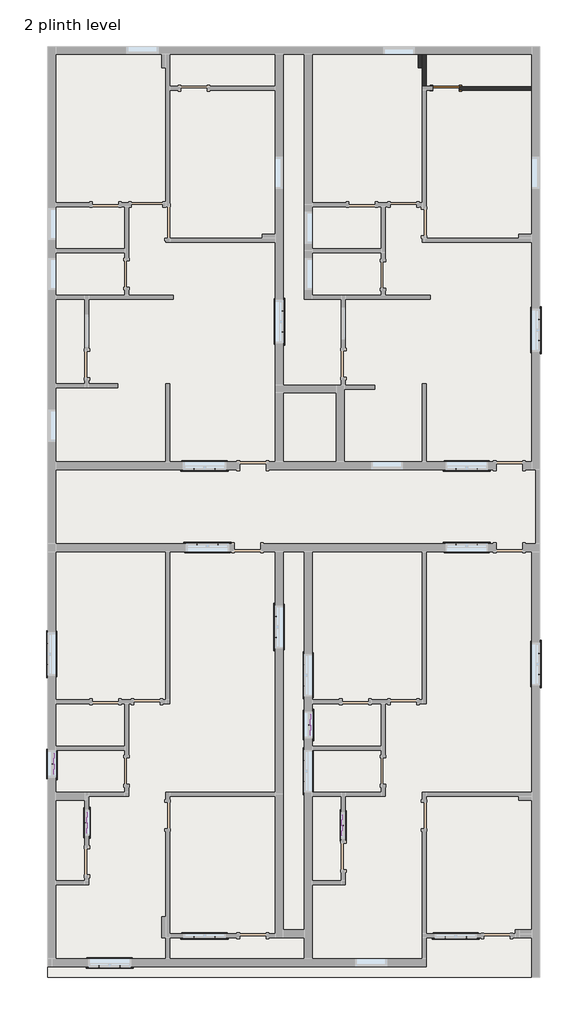
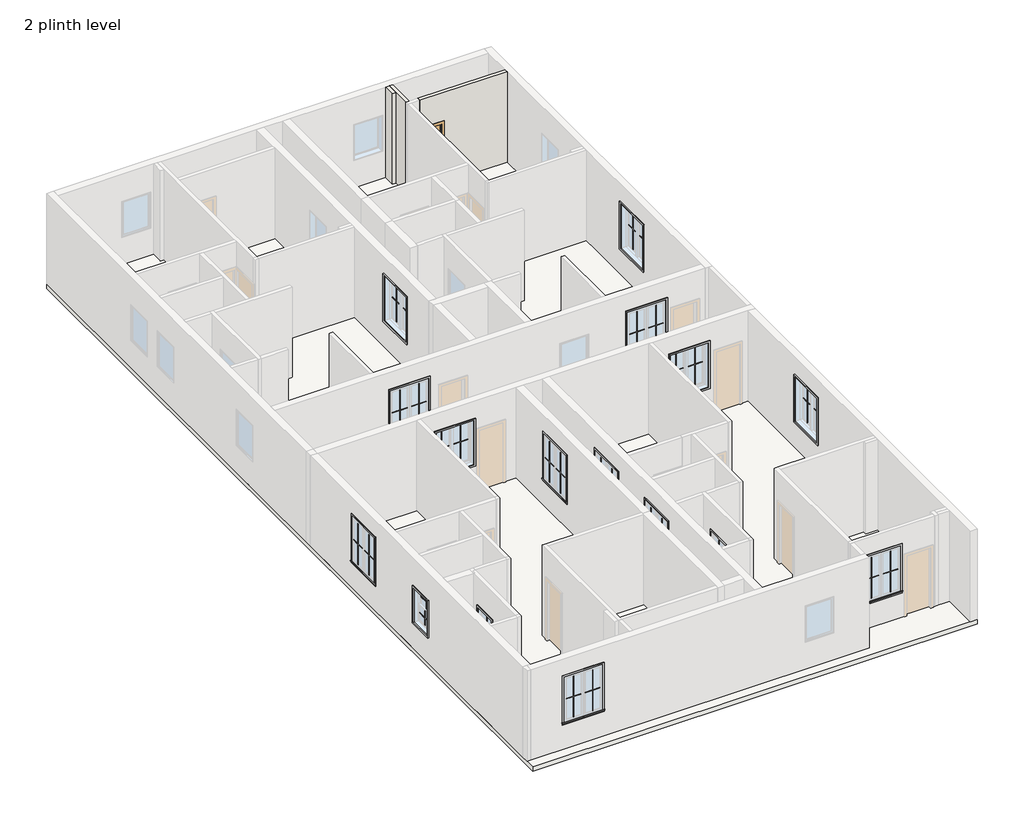
# One storey, part 4 of 4: 72 proxies, 3 walls, 1 door, 1 slab.
"""IFC4 building model written with IfcOpenShell, lengths in millimetres."""

from ifc_helpers import new_model, si_unit, frame, origin, place, context, project, spatial, polyline, outline, extrude, faceted_brep, transform, mapped, element, save
from components import muntin_pattern_2x2_muntin_pattern_2x2_6dad3731, muntin_pattern_2x2_muntin_pattern_2x2_a30a3345, muntin_pattern_2x2_muntin_pattern_2x2_b8ba09c9, trim_window_exterior_flat_with_sill_92b9b949, trim_window_exterior_flat_with_sill_6cd3ad68, trim_window_interior_flat_picture_frame_3bb882cf, trim_window_interior_flat_picture_frame_840a62db, door_f2b275c1

model = new_model("IFC4")

# Units and contexts
model_context = context("Model", 3, world=origin())
ifc_project = project(units=[si_unit("LENGTHUNIT", "METRE", prefix="MILLI")], contexts=[model_context])

# Site, building, storey
site = spatial("IfcSite", under=ifc_project)
building = spatial("IfcBuilding", under=site)
storey = spatial("IfcBuildingStorey", under=building, Name="2 plinth level", Elevation=457.2)

# Proxies
placement = place(None, origin())
muntin_pattern_2x2_muntin_pattern_2x2_shape = muntin_pattern_2x2_muntin_pattern_2x2_6dad3731(model_context)
element("IfcBuildingElementProxy", 1, Name="Muntin Pattern_2x2 : Muntin Pattern_2x2", ObjectType="Muntin Pattern_2x2 : Muntin Pattern_2x2", at=placement, inside=storey, context=model_context, shape_type="MappedRepresentation", body=[
    mapped(muntin_pattern_2x2_muntin_pattern_2x2_shape, transform((-8343.3525468, -3788.9429449, 1441.45), x_axis=(0.0, 1.0, 0.0), y_axis=(-1.0, 0.0, 0.0), z_axis=(0.0, 0.0, 1.0))),
])
element("IfcBuildingElementProxy", 2, Name="Muntin Pattern_2x2 : Muntin Pattern_2x2", ObjectType="Muntin Pattern_2x2 : Muntin Pattern_2x2", at=placement, inside=storey, context=model_context, shape_type="MappedRepresentation", body=[
    mapped(muntin_pattern_2x2_muntin_pattern_2x2_shape, transform((-4055.5150468, -313.9054449, 1441.45), x_axis=(1.0, 0.0, 0.0), y_axis=(0.0, 1.0, 0.0), z_axis=(0.0, 0.0, 1.0))),
])
element("IfcBuildingElementProxy", 3, Name="Muntin Pattern_2x2 : Muntin Pattern_2x2", ObjectType="Muntin Pattern_2x2 : Muntin Pattern_2x2", at=placement, inside=storey, context=model_context, shape_type="MappedRepresentation", body=[
    mapped(muntin_pattern_2x2_muntin_pattern_2x2_shape, transform((3412.0849532, -313.9054449, 1441.45), x_axis=(1.0, 0.0, 0.0), y_axis=(0.0, 1.0, 0.0), z_axis=(0.0, 0.0, 1.0))),
])
element("IfcBuildingElementProxy", 4, Name="Muntin Pattern_2x2 : Muntin Pattern_2x2", ObjectType="Muntin Pattern_2x2 : Muntin Pattern_2x2", at=placement, inside=storey, context=model_context, shape_type="MappedRepresentation", body=[
    mapped(muntin_pattern_2x2_muntin_pattern_2x2_shape, transform((5810.7974532, -3468.2679449, 1441.45), x_axis=(0.0, -1.0, 0.0), y_axis=(1.0, 0.0, 0.0), z_axis=(0.0, 0.0, 1.0))),
])
element("IfcBuildingElementProxy", 5, Name="Muntin Pattern_2x2 : Muntin Pattern_2x2", ObjectType="Muntin Pattern_2x2 : Muntin Pattern_2x2", at=placement, inside=storey, context=model_context, shape_type="MappedRepresentation", body=[
    mapped(muntin_pattern_2x2_muntin_pattern_2x2_shape, transform((-1790.1525468, -3007.8929449, 1441.45), x_axis=(0.0, 1.0, 0.0), y_axis=(-1.0, 0.0, 0.0), z_axis=(0.0, 0.0, 1.0))),
])
element("IfcBuildingElementProxy", 6, Name="Muntin Pattern_2x2 : Muntin Pattern_2x2", ObjectType="Muntin Pattern_2x2 : Muntin Pattern_2x2", at=placement, inside=storey, context=model_context, shape_type="MappedRepresentation", body=[
    mapped(muntin_pattern_2x2_muntin_pattern_2x2_shape, transform((-951.9525468, -4398.5429449, 1441.45), x_axis=(0.0, 1.0, 0.0), y_axis=(-1.0, 0.0, 0.0), z_axis=(0.0, 0.0, 1.0))),
])
element("IfcBuildingElementProxy", 7, Name="Muntin Pattern_2x2 : Muntin Pattern_2x2", ObjectType="Muntin Pattern_2x2 : Muntin Pattern_2x2", at=placement, inside=storey, context=model_context, shape_type="MappedRepresentation", body=[
    mapped(muntin_pattern_2x2_muntin_pattern_2x2_shape, transform((-3534.8150468, 1838.7445552, 1441.45), x_axis=(-1.0, 0.0, 0.0), y_axis=(0.0, -1.0, 0.0), z_axis=(0.0, 0.0, 1.0))),
])
element("IfcBuildingElementProxy", 8, Name="Muntin Pattern_2x2 : Muntin Pattern_2x2", ObjectType="Muntin Pattern_2x2 : Muntin Pattern_2x2", at=placement, inside=storey, context=model_context, shape_type="MappedRepresentation", body=[
    mapped(muntin_pattern_2x2_muntin_pattern_2x2_shape, transform((4018.5099532, 1838.7445552, 1441.45), x_axis=(-1.0, 0.0, 0.0), y_axis=(0.0, -1.0, 0.0), z_axis=(0.0, 0.0, 1.0))),
])
element("IfcBuildingElementProxy", 9, Name="Muntin Pattern_2x2 : Muntin Pattern_2x2", ObjectType="Muntin Pattern_2x2 : Muntin Pattern_2x2", at=placement, inside=storey, context=model_context, shape_type="MappedRepresentation", body=[
    mapped(muntin_pattern_2x2_muntin_pattern_2x2_shape, transform((5810.7974532, 6151.9820551, 1441.45), x_axis=(0.0, -1.0, 0.0), y_axis=(1.0, 0.0, 0.0), z_axis=(0.0, 0.0, 1.0))),
])
element("IfcBuildingElementProxy", 10, Name="Muntin Pattern_2x2 : Muntin Pattern_2x2", ObjectType="Muntin Pattern_2x2 : Muntin Pattern_2x2", at=placement, inside=storey, context=model_context, shape_type="MappedRepresentation", body=[
    mapped(muntin_pattern_2x2_muntin_pattern_2x2_shape, transform((-1580.6025468, 6399.6320551, 1441.45), x_axis=(0.0, -1.0, 0.0), y_axis=(1.0, 0.0, 0.0), z_axis=(0.0, 0.0, 1.0))),
])
element("IfcBuildingElementProxy", 11, Name="Muntin Pattern_2x2 : Muntin Pattern_2x2", ObjectType="Muntin Pattern_2x2 : Muntin Pattern_2x2", at=placement, inside=storey, context=model_context, shape_type="MappedRepresentation", body=[
    mapped(muntin_pattern_2x2_muntin_pattern_2x2_shape, transform((-951.9525468, -7160.7929449, 1441.45), x_axis=(0.0, 1.0, 0.0), y_axis=(-1.0, 0.0, 0.0), z_axis=(0.0, 0.0, 1.0))),
])
element("IfcBuildingElementProxy", 12, Name="Muntin Pattern_2x2 : Muntin Pattern_2x2", ObjectType="Muntin Pattern_2x2 : Muntin Pattern_2x2", at=placement, inside=storey, context=model_context, shape_type="MappedRepresentation", body=[
    mapped(muntin_pattern_2x2_muntin_pattern_2x2_shape, transform((-6268.4900468, -12486.8554449, 1441.45), x_axis=(-1.0, 0.0, 0.0), y_axis=(0.0, -1.0, 0.0), z_axis=(0.0, 0.0, 1.0))),
])
element("IfcBuildingElementProxy", 13, Name="Muntin Pattern_2x2 : Muntin Pattern_2x2", ObjectType="Muntin Pattern_2x2 : Muntin Pattern_2x2", at=placement, inside=storey, context=model_context, shape_type="MappedRepresentation", body=[
    mapped(muntin_pattern_2x2_muntin_pattern_2x2_shape, transform((-3534.8150468, -11648.6554449, 1441.45), x_axis=(-1.0, 0.0, 0.0), y_axis=(0.0, -1.0, 0.0), z_axis=(0.0, 0.0, 1.0))),
])
element("IfcBuildingElementProxy", 14, Name="Muntin Pattern_2x2 : Muntin Pattern_2x2", ObjectType="Muntin Pattern_2x2 : Muntin Pattern_2x2", at=placement, inside=storey, context=model_context, shape_type="MappedRepresentation", body=[
    mapped(muntin_pattern_2x2_muntin_pattern_2x2_shape, transform((3703.5438613, -11651.7034449, 1441.45), x_axis=(-1.0, 0.0, 0.0), y_axis=(0.0, -1.0, 0.0), z_axis=(0.0, 0.0, 1.0))),
])
muntin_pattern_2x2_muntin_pattern_2x2_2_shape = muntin_pattern_2x2_muntin_pattern_2x2_a30a3345(model_context)
element("IfcBuildingElementProxy", 15, Name="Muntin Pattern_2x2 : Muntin Pattern_2x2", ObjectType="Muntin Pattern_2x2 : Muntin Pattern_2x2", at=placement, inside=storey, context=model_context, shape_type="MappedRepresentation", body=[
    mapped(muntin_pattern_2x2_muntin_pattern_2x2_2_shape, transform((-8343.3525468, -3182.5179449, 1441.45), x_axis=(0.0, -1.0, 0.0), y_axis=(1.0, 0.0, 0.0), z_axis=(0.0, 0.0, 1.0))),
])
element("IfcBuildingElementProxy", 16, Name="Muntin Pattern_2x2 : Muntin Pattern_2x2", ObjectType="Muntin Pattern_2x2 : Muntin Pattern_2x2", at=placement, inside=storey, context=model_context, shape_type="MappedRepresentation", body=[
    mapped(muntin_pattern_2x2_muntin_pattern_2x2_2_shape, transform((-3449.0900468, -313.9054449, 1441.45), x_axis=(-1.0, 0.0, 0.0), y_axis=(0.0, -1.0, 0.0), z_axis=(0.0, 0.0, 1.0))),
])
element("IfcBuildingElementProxy", 17, Name="Muntin Pattern_2x2 : Muntin Pattern_2x2", ObjectType="Muntin Pattern_2x2 : Muntin Pattern_2x2", at=placement, inside=storey, context=model_context, shape_type="MappedRepresentation", body=[
    mapped(muntin_pattern_2x2_muntin_pattern_2x2_2_shape, transform((4018.5099532, -313.9054449, 1441.45), x_axis=(-1.0, 0.0, 0.0), y_axis=(0.0, -1.0, 0.0), z_axis=(0.0, 0.0, 1.0))),
])
element("IfcBuildingElementProxy", 18, Name="Muntin Pattern_2x2 : Muntin Pattern_2x2", ObjectType="Muntin Pattern_2x2 : Muntin Pattern_2x2", at=placement, inside=storey, context=model_context, shape_type="MappedRepresentation", body=[
    mapped(muntin_pattern_2x2_muntin_pattern_2x2_2_shape, transform((5810.7974532, -4074.6929449, 1441.45), x_axis=(0.0, 1.0, 0.0), y_axis=(-1.0, 0.0, 0.0), z_axis=(0.0, 0.0, 1.0))),
])
element("IfcBuildingElementProxy", 19, Name="Muntin Pattern_2x2 : Muntin Pattern_2x2", ObjectType="Muntin Pattern_2x2 : Muntin Pattern_2x2", at=placement, inside=storey, context=model_context, shape_type="MappedRepresentation", body=[
    mapped(muntin_pattern_2x2_muntin_pattern_2x2_2_shape, transform((-1790.1525468, -2401.4679449, 1441.45), x_axis=(0.0, -1.0, 0.0), y_axis=(1.0, 0.0, 0.0), z_axis=(0.0, 0.0, 1.0))),
])
element("IfcBuildingElementProxy", 20, Name="Muntin Pattern_2x2 : Muntin Pattern_2x2", ObjectType="Muntin Pattern_2x2 : Muntin Pattern_2x2", at=placement, inside=storey, context=model_context, shape_type="MappedRepresentation", body=[
    mapped(muntin_pattern_2x2_muntin_pattern_2x2_2_shape, transform((-951.9525468, -3792.1179449, 1441.45), x_axis=(0.0, -1.0, 0.0), y_axis=(1.0, 0.0, 0.0), z_axis=(0.0, 0.0, 1.0))),
])
element("IfcBuildingElementProxy", 21, Name="Muntin Pattern_2x2 : Muntin Pattern_2x2", ObjectType="Muntin Pattern_2x2 : Muntin Pattern_2x2", at=placement, inside=storey, context=model_context, shape_type="MappedRepresentation", body=[
    mapped(muntin_pattern_2x2_muntin_pattern_2x2_2_shape, transform((-4141.2400468, 1838.7445552, 1441.45), x_axis=(1.0, 0.0, 0.0), y_axis=(0.0, 1.0, 0.0), z_axis=(0.0, 0.0, 1.0))),
])
element("IfcBuildingElementProxy", 22, Name="Muntin Pattern_2x2 : Muntin Pattern_2x2", ObjectType="Muntin Pattern_2x2 : Muntin Pattern_2x2", at=placement, inside=storey, context=model_context, shape_type="MappedRepresentation", body=[
    mapped(muntin_pattern_2x2_muntin_pattern_2x2_2_shape, transform((3412.0849532, 1838.7445552, 1441.45), x_axis=(1.0, 0.0, 0.0), y_axis=(0.0, 1.0, 0.0), z_axis=(0.0, 0.0, 1.0))),
])
element("IfcBuildingElementProxy", 23, Name="Muntin Pattern_2x2 : Muntin Pattern_2x2", ObjectType="Muntin Pattern_2x2 : Muntin Pattern_2x2", at=placement, inside=storey, context=model_context, shape_type="MappedRepresentation", body=[
    mapped(muntin_pattern_2x2_muntin_pattern_2x2_2_shape, transform((5810.7974532, 5545.5570551, 1441.45), x_axis=(0.0, 1.0, 0.0), y_axis=(-1.0, 0.0, 0.0), z_axis=(0.0, 0.0, 1.0))),
])
element("IfcBuildingElementProxy", 24, Name="Muntin Pattern_2x2 : Muntin Pattern_2x2", ObjectType="Muntin Pattern_2x2 : Muntin Pattern_2x2", at=placement, inside=storey, context=model_context, shape_type="MappedRepresentation", body=[
    mapped(muntin_pattern_2x2_muntin_pattern_2x2_2_shape, transform((-1580.6025468, 5793.2070551, 1441.45), x_axis=(0.0, 1.0, 0.0), y_axis=(-1.0, 0.0, 0.0), z_axis=(0.0, 0.0, 1.0))),
])
element("IfcBuildingElementProxy", 25, Name="Muntin Pattern_2x2 : Muntin Pattern_2x2", ObjectType="Muntin Pattern_2x2 : Muntin Pattern_2x2", at=placement, inside=storey, context=model_context, shape_type="MappedRepresentation", body=[
    mapped(muntin_pattern_2x2_muntin_pattern_2x2_2_shape, transform((-951.9525468, -6554.3679449, 1441.45), x_axis=(0.0, -1.0, 0.0), y_axis=(1.0, 0.0, 0.0), z_axis=(0.0, 0.0, 1.0))),
])
element("IfcBuildingElementProxy", 26, Name="Muntin Pattern_2x2 : Muntin Pattern_2x2", ObjectType="Muntin Pattern_2x2 : Muntin Pattern_2x2", at=placement, inside=storey, context=model_context, shape_type="MappedRepresentation", body=[
    mapped(muntin_pattern_2x2_muntin_pattern_2x2_2_shape, transform((-6874.9150468, -12486.8554449, 1441.45), x_axis=(1.0, 0.0, 0.0), y_axis=(0.0, 1.0, 0.0), z_axis=(0.0, 0.0, 1.0))),
])
element("IfcBuildingElementProxy", 27, Name="Muntin Pattern_2x2 : Muntin Pattern_2x2", ObjectType="Muntin Pattern_2x2 : Muntin Pattern_2x2", at=placement, inside=storey, context=model_context, shape_type="MappedRepresentation", body=[
    mapped(muntin_pattern_2x2_muntin_pattern_2x2_2_shape, transform((-4141.2400468, -11648.6554449, 1441.45), x_axis=(1.0, 0.0, 0.0), y_axis=(0.0, 1.0, 0.0), z_axis=(0.0, 0.0, 1.0))),
])
element("IfcBuildingElementProxy", 28, Name="Muntin Pattern_2x2 : Muntin Pattern_2x2", ObjectType="Muntin Pattern_2x2 : Muntin Pattern_2x2", at=placement, inside=storey, context=model_context, shape_type="MappedRepresentation", body=[
    mapped(muntin_pattern_2x2_muntin_pattern_2x2_2_shape, transform((3097.1188613, -11651.7034449, 1441.45), x_axis=(1.0, 0.0, 0.0), y_axis=(0.0, 1.0, 0.0), z_axis=(0.0, 0.0, 1.0))),
])
muntin_pattern_2x2_muntin_pattern_2x2_3_shape = muntin_pattern_2x2_muntin_pattern_2x2_b8ba09c9(model_context)
element("IfcBuildingElementProxy", 29, Name="Muntin Pattern_2x2 : Muntin Pattern_2x2", ObjectType="Muntin Pattern_2x2 : Muntin Pattern_2x2", at=placement, inside=storey, context=model_context, shape_type="MappedRepresentation", body=[
    mapped(muntin_pattern_2x2_muntin_pattern_2x2_3_shape, transform((-8159.2025468, -6648.0304448, 1978.025), x_axis=(0.0, -1.0, 0.0), y_axis=(1.0, 0.0, 0.0), z_axis=(0.0, 0.0, 1.0))),
])
element("IfcBuildingElementProxy", 30, Name="Muntin Pattern_2x2 : Muntin Pattern_2x2", ObjectType="Muntin Pattern_2x2 : Muntin Pattern_2x2", at=placement, inside=storey, context=model_context, shape_type="MappedRepresentation", body=[
    mapped(muntin_pattern_2x2_muntin_pattern_2x2_3_shape, transform((-8203.6525468, -6648.0304448, 1447.8), x_axis=(0.0, -1.0, 0.0), y_axis=(1.0, 0.0, 0.0), z_axis=(0.0, 0.0, 1.0))),
])
element("IfcBuildingElementProxy", 31, Name="Muntin Pattern_2x2 : Muntin Pattern_2x2", ObjectType="Muntin Pattern_2x2 : Muntin Pattern_2x2", at=placement, inside=storey, context=model_context, shape_type="MappedRepresentation", body=[
    mapped(muntin_pattern_2x2_muntin_pattern_2x2_3_shape, transform((-767.8025468, -5524.0804449, 1978.025), x_axis=(0.0, -1.0, 0.0), y_axis=(1.0, 0.0, 0.0), z_axis=(0.0, 0.0, 1.0))),
])
element("IfcBuildingElementProxy", 32, Name="Muntin Pattern_2x2 : Muntin Pattern_2x2", ObjectType="Muntin Pattern_2x2 : Muntin Pattern_2x2", at=placement, inside=storey, context=model_context, shape_type="MappedRepresentation", body=[
    mapped(muntin_pattern_2x2_muntin_pattern_2x2_3_shape, transform((-812.2525468, -5524.0804449, 1447.8), x_axis=(0.0, -1.0, 0.0), y_axis=(1.0, 0.0, 0.0), z_axis=(0.0, 0.0, 1.0))),
])
element("IfcBuildingElementProxy", 33, Name="Muntin Pattern_2x2 : Muntin Pattern_2x2", ObjectType="Muntin Pattern_2x2 : Muntin Pattern_2x2", at=placement, inside=storey, context=model_context, shape_type="MappedRepresentation", body=[
    mapped(muntin_pattern_2x2_muntin_pattern_2x2_3_shape, transform((-7206.7025468, -8343.4804449, 1978.025), x_axis=(0.0, -1.0, 0.0), y_axis=(1.0, 0.0, 0.0), z_axis=(0.0, 0.0, 1.0))),
])
element("IfcBuildingElementProxy", 34, Name="Muntin Pattern_2x2 : Muntin Pattern_2x2", ObjectType="Muntin Pattern_2x2 : Muntin Pattern_2x2", at=placement, inside=storey, context=model_context, shape_type="MappedRepresentation", body=[
    mapped(muntin_pattern_2x2_muntin_pattern_2x2_3_shape, transform((-7251.1525468, -8343.4804449, 1447.8), x_axis=(0.0, -1.0, 0.0), y_axis=(1.0, 0.0, 0.0), z_axis=(0.0, 0.0, 1.0))),
])
element("IfcBuildingElementProxy", 35, Name="Muntin Pattern_2x2 : Muntin Pattern_2x2", ObjectType="Muntin Pattern_2x2 : Muntin Pattern_2x2", at=placement, inside=storey, context=model_context, shape_type="MappedRepresentation", body=[
    mapped(muntin_pattern_2x2_muntin_pattern_2x2_3_shape, transform((140.2474532, -8419.6804449, 1978.025), x_axis=(0.0, 1.0, 0.0), y_axis=(-1.0, 0.0, 0.0), z_axis=(0.0, 0.0, 1.0))),
])
element("IfcBuildingElementProxy", 36, Name="Muntin Pattern_2x2 : Muntin Pattern_2x2", ObjectType="Muntin Pattern_2x2 : Muntin Pattern_2x2", at=placement, inside=storey, context=model_context, shape_type="MappedRepresentation", body=[
    mapped(muntin_pattern_2x2_muntin_pattern_2x2_3_shape, transform((184.6974532, -8419.6804449, 1447.8), x_axis=(0.0, 1.0, 0.0), y_axis=(-1.0, 0.0, 0.0), z_axis=(0.0, 0.0, 1.0))),
])
trim_window_exterior_flat_with_sill_shape = trim_window_exterior_flat_with_sill_92b9b949(model_context)
element("IfcBuildingElementProxy", 37, Name="Trim-Window-Exterior-Flat : with Sill", ObjectType="Trim-Window-Exterior-Flat : with Sill", at=placement, inside=storey, context=model_context, shape_type="MappedRepresentation", body=[
    mapped(trim_window_exterior_flat_with_sill_shape, transform((-8352.8775468, -3485.7304449, 2895.6), x_axis=(0.0, -1.0, 0.0), y_axis=(0.0, 0.0, 1.0), z_axis=(-1.0, 0.0, 0.0))),
])
element("IfcBuildingElementProxy", 38, Name="Trim-Window-Exterior-Flat : with Sill", ObjectType="Trim-Window-Exterior-Flat : with Sill", at=placement, inside=storey, context=model_context, shape_type="MappedRepresentation", body=[
    mapped(trim_window_exterior_flat_with_sill_shape, transform((-3752.3025468, -304.3804449, 2895.6), x_axis=(-1.0, 0.0, 0.0), y_axis=(0.0, 0.0, 1.0), z_axis=(0.0, 1.0, 0.0))),
])
element("IfcBuildingElementProxy", 39, Name="Trim-Window-Exterior-Flat : with Sill", ObjectType="Trim-Window-Exterior-Flat : with Sill", at=placement, inside=storey, context=model_context, shape_type="MappedRepresentation", body=[
    mapped(trim_window_exterior_flat_with_sill_shape, transform((3715.2974532, -304.3804449, 2895.6), x_axis=(-1.0, 0.0, 0.0), y_axis=(0.0, 0.0, 1.0), z_axis=(0.0, 1.0, 0.0))),
])
element("IfcBuildingElementProxy", 40, Name="Trim-Window-Exterior-Flat : with Sill", ObjectType="Trim-Window-Exterior-Flat : with Sill", at=placement, inside=storey, context=model_context, shape_type="MappedRepresentation", body=[
    mapped(trim_window_exterior_flat_with_sill_shape, transform((5820.3224532, -3771.4804449, 2895.6), x_axis=(0.0, 1.0, 0.0), y_axis=(0.0, 0.0, 1.0), z_axis=(1.0, 0.0, 0.0))),
])
element("IfcBuildingElementProxy", 41, Name="Trim-Window-Exterior-Flat : with Sill", ObjectType="Trim-Window-Exterior-Flat : with Sill", at=placement, inside=storey, context=model_context, shape_type="MappedRepresentation", body=[
    mapped(trim_window_exterior_flat_with_sill_shape, transform((-1799.6775468, -2704.6804449, 2895.6), x_axis=(0.0, -1.0, 0.0), y_axis=(0.0, 0.0, 1.0), z_axis=(-1.0, 0.0, 0.0))),
])
element("IfcBuildingElementProxy", 42, Name="Trim-Window-Exterior-Flat : with Sill", ObjectType="Trim-Window-Exterior-Flat : with Sill", at=placement, inside=storey, context=model_context, shape_type="MappedRepresentation", body=[
    mapped(trim_window_exterior_flat_with_sill_shape, transform((-961.4775468, -4095.3304449, 2895.6), x_axis=(0.0, -1.0, 0.0), y_axis=(0.0, 0.0, 1.0), z_axis=(-1.0, 0.0, 0.0))),
])
element("IfcBuildingElementProxy", 43, Name="Trim-Window-Exterior-Flat : with Sill", ObjectType="Trim-Window-Exterior-Flat : with Sill", at=placement, inside=storey, context=model_context, shape_type="MappedRepresentation", body=[
    mapped(trim_window_exterior_flat_with_sill_shape, transform((-3838.0275468, 1829.2195552, 2895.6), x_axis=(1.0, 0.0, 0.0), y_axis=(0.0, 0.0, 1.0), z_axis=(0.0, -1.0, 0.0))),
])
element("IfcBuildingElementProxy", 44, Name="Trim-Window-Exterior-Flat : with Sill", ObjectType="Trim-Window-Exterior-Flat : with Sill", at=placement, inside=storey, context=model_context, shape_type="MappedRepresentation", body=[
    mapped(trim_window_exterior_flat_with_sill_shape, transform((3715.2974532, 1829.2195552, 2895.6), x_axis=(1.0, 0.0, 0.0), y_axis=(0.0, 0.0, 1.0), z_axis=(0.0, -1.0, 0.0))),
])
element("IfcBuildingElementProxy", 45, Name="Trim-Window-Exterior-Flat : with Sill", ObjectType="Trim-Window-Exterior-Flat : with Sill", at=placement, inside=storey, context=model_context, shape_type="MappedRepresentation", body=[
    mapped(trim_window_exterior_flat_with_sill_shape, transform((5820.3224532, 5848.7695551, 2895.6), x_axis=(0.0, 1.0, 0.0), y_axis=(0.0, 0.0, 1.0), z_axis=(1.0, 0.0, 0.0))),
])
element("IfcBuildingElementProxy", 46, Name="Trim-Window-Exterior-Flat : with Sill", ObjectType="Trim-Window-Exterior-Flat : with Sill", at=placement, inside=storey, context=model_context, shape_type="MappedRepresentation", body=[
    mapped(trim_window_exterior_flat_with_sill_shape, transform((-1571.0775468, 6096.4195551, 2895.6), x_axis=(0.0, 1.0, 0.0), y_axis=(0.0, 0.0, 1.0), z_axis=(1.0, 0.0, 0.0))),
])
element("IfcBuildingElementProxy", 47, Name="Trim-Window-Exterior-Flat : with Sill", ObjectType="Trim-Window-Exterior-Flat : with Sill", at=placement, inside=storey, context=model_context, shape_type="MappedRepresentation", body=[
    mapped(trim_window_exterior_flat_with_sill_shape, transform((-961.4775468, -6857.5804449, 2895.6), x_axis=(0.0, -1.0, 0.0), y_axis=(0.0, 0.0, 1.0), z_axis=(-1.0, 0.0, 0.0))),
])
element("IfcBuildingElementProxy", 48, Name="Trim-Window-Exterior-Flat : with Sill", ObjectType="Trim-Window-Exterior-Flat : with Sill", at=placement, inside=storey, context=model_context, shape_type="MappedRepresentation", body=[
    mapped(trim_window_exterior_flat_with_sill_shape, transform((-6571.7025468, -12496.3804449, 2895.6), x_axis=(1.0, 0.0, 0.0), y_axis=(0.0, 0.0, 1.0), z_axis=(0.0, -1.0, 0.0))),
])
element("IfcBuildingElementProxy", 49, Name="Trim-Window-Exterior-Flat : with Sill", ObjectType="Trim-Window-Exterior-Flat : with Sill", at=placement, inside=storey, context=model_context, shape_type="MappedRepresentation", body=[
    mapped(trim_window_exterior_flat_with_sill_shape, transform((-3838.0275468, -11658.1804449, 2895.6), x_axis=(1.0, 0.0, 0.0), y_axis=(0.0, 0.0, 1.0), z_axis=(0.0, -1.0, 0.0))),
])
element("IfcBuildingElementProxy", 50, Name="Trim-Window-Exterior-Flat : with Sill", ObjectType="Trim-Window-Exterior-Flat : with Sill", at=placement, inside=storey, context=model_context, shape_type="MappedRepresentation", body=[
    mapped(trim_window_exterior_flat_with_sill_shape, transform((3400.3313613, -11661.2284449, 2895.6), x_axis=(1.0, 0.0, 0.0), y_axis=(0.0, 0.0, 1.0), z_axis=(0.0, -1.0, 0.0))),
])
trim_window_exterior_flat_with_sill_2_shape = trim_window_exterior_flat_with_sill_6cd3ad68(model_context)
element("IfcBuildingElementProxy", 51, Name="Trim-Window-Exterior-Flat : with Sill", ObjectType="Trim-Window-Exterior-Flat : with Sill", at=placement, inside=storey, context=model_context, shape_type="MappedRepresentation", body=[
    mapped(trim_window_exterior_flat_with_sill_2_shape, transform((-8124.2775468, -6648.0304448, 2540.0), x_axis=(0.0, 1.0, 0.0), y_axis=(0.0, 0.0, 1.0), z_axis=(1.0, 0.0, 0.0))),
])
element("IfcBuildingElementProxy", 52, Name="Trim-Window-Exterior-Flat : with Sill", ObjectType="Trim-Window-Exterior-Flat : with Sill", at=placement, inside=storey, context=model_context, shape_type="MappedRepresentation", body=[
    mapped(trim_window_exterior_flat_with_sill_2_shape, transform((-732.8775468, -5524.0804449, 2540.0), x_axis=(0.0, 1.0, 0.0), y_axis=(0.0, 0.0, 1.0), z_axis=(1.0, 0.0, 0.0))),
])
element("IfcBuildingElementProxy", 53, Name="Trim-Window-Exterior-Flat : with Sill", ObjectType="Trim-Window-Exterior-Flat : with Sill", at=placement, inside=storey, context=model_context, shape_type="MappedRepresentation", body=[
    mapped(trim_window_exterior_flat_with_sill_2_shape, transform((-7171.7775468, -8343.4804449, 2540.0), x_axis=(0.0, 1.0, 0.0), y_axis=(0.0, 0.0, 1.0), z_axis=(1.0, 0.0, 0.0))),
])
element("IfcBuildingElementProxy", 54, Name="Trim-Window-Exterior-Flat : with Sill", ObjectType="Trim-Window-Exterior-Flat : with Sill", at=placement, inside=storey, context=model_context, shape_type="MappedRepresentation", body=[
    mapped(trim_window_exterior_flat_with_sill_2_shape, transform((105.3224532, -8419.6804449, 2540.0), x_axis=(0.0, -1.0, 0.0), y_axis=(0.0, 0.0, 1.0), z_axis=(-1.0, 0.0, 0.0))),
])
trim_window_interior_flat_picture_frame_shape = trim_window_interior_flat_picture_frame_3bb882cf(model_context)
element("IfcBuildingElementProxy", 55, Name="Trim-Window-Interior-Flat : Picture Frame", ObjectType="Trim-Window-Interior-Flat : Picture Frame", at=placement, inside=storey, context=model_context, shape_type="MappedRepresentation", body=[
    mapped(trim_window_interior_flat_picture_frame_shape, transform((-8124.2775468, -3485.7304449, 2895.6), x_axis=(0.0, 1.0, 0.0), y_axis=(0.0, 0.0, 1.0), z_axis=(1.0, 0.0, 0.0))),
])
element("IfcBuildingElementProxy", 56, Name="Trim-Window-Interior-Flat : Picture Frame", ObjectType="Trim-Window-Interior-Flat : Picture Frame", at=placement, inside=storey, context=model_context, shape_type="MappedRepresentation", body=[
    mapped(trim_window_interior_flat_picture_frame_shape, transform((-3752.3025468, -532.9804449, 2895.6), x_axis=(1.0, 0.0, 0.0), y_axis=(0.0, 0.0, 1.0), z_axis=(0.0, -1.0, 0.0))),
])
element("IfcBuildingElementProxy", 57, Name="Trim-Window-Interior-Flat : Picture Frame", ObjectType="Trim-Window-Interior-Flat : Picture Frame", at=placement, inside=storey, context=model_context, shape_type="MappedRepresentation", body=[
    mapped(trim_window_interior_flat_picture_frame_shape, transform((3715.2974532, -532.9804449, 2895.6), x_axis=(1.0, 0.0, 0.0), y_axis=(0.0, 0.0, 1.0), z_axis=(0.0, -1.0, 0.0))),
])
element("IfcBuildingElementProxy", 58, Name="Trim-Window-Interior-Flat : Picture Frame", ObjectType="Trim-Window-Interior-Flat : Picture Frame", at=placement, inside=storey, context=model_context, shape_type="MappedRepresentation", body=[
    mapped(trim_window_interior_flat_picture_frame_shape, transform((5591.7224532, -3771.4804449, 2895.6), x_axis=(0.0, -1.0, 0.0), y_axis=(0.0, 0.0, 1.0), z_axis=(-1.0, 0.0, 0.0))),
])
element("IfcBuildingElementProxy", 59, Name="Trim-Window-Interior-Flat : Picture Frame", ObjectType="Trim-Window-Interior-Flat : Picture Frame", at=placement, inside=storey, context=model_context, shape_type="MappedRepresentation", body=[
    mapped(trim_window_interior_flat_picture_frame_shape, transform((-1571.0775468, -2704.6804449, 2895.6), x_axis=(0.0, 1.0, 0.0), y_axis=(0.0, 0.0, 1.0), z_axis=(1.0, 0.0, 0.0))),
])
element("IfcBuildingElementProxy", 60, Name="Trim-Window-Interior-Flat : Picture Frame", ObjectType="Trim-Window-Interior-Flat : Picture Frame", at=placement, inside=storey, context=model_context, shape_type="MappedRepresentation", body=[
    mapped(trim_window_interior_flat_picture_frame_shape, transform((-732.8775468, -4095.3304449, 2895.6), x_axis=(0.0, 1.0, 0.0), y_axis=(0.0, 0.0, 1.0), z_axis=(1.0, 0.0, 0.0))),
])
element("IfcBuildingElementProxy", 61, Name="Trim-Window-Interior-Flat : Picture Frame", ObjectType="Trim-Window-Interior-Flat : Picture Frame", at=placement, inside=storey, context=model_context, shape_type="MappedRepresentation", body=[
    mapped(trim_window_interior_flat_picture_frame_shape, transform((-3838.0275468, 2057.8195552, 2895.6), x_axis=(-1.0, 0.0, 0.0), y_axis=(0.0, 0.0, 1.0), z_axis=(0.0, 1.0, 0.0))),
])
element("IfcBuildingElementProxy", 62, Name="Trim-Window-Interior-Flat : Picture Frame", ObjectType="Trim-Window-Interior-Flat : Picture Frame", at=placement, inside=storey, context=model_context, shape_type="MappedRepresentation", body=[
    mapped(trim_window_interior_flat_picture_frame_shape, transform((3715.2974532, 2057.8195552, 2895.6), x_axis=(-1.0, 0.0, 0.0), y_axis=(0.0, 0.0, 1.0), z_axis=(0.0, 1.0, 0.0))),
])
element("IfcBuildingElementProxy", 63, Name="Trim-Window-Interior-Flat : Picture Frame", ObjectType="Trim-Window-Interior-Flat : Picture Frame", at=placement, inside=storey, context=model_context, shape_type="MappedRepresentation", body=[
    mapped(trim_window_interior_flat_picture_frame_shape, transform((5591.7224532, 5848.7695551, 2895.6), x_axis=(0.0, -1.0, 0.0), y_axis=(0.0, 0.0, 1.0), z_axis=(-1.0, 0.0, 0.0))),
])
element("IfcBuildingElementProxy", 64, Name="Trim-Window-Interior-Flat : Picture Frame", ObjectType="Trim-Window-Interior-Flat : Picture Frame", at=placement, inside=storey, context=model_context, shape_type="MappedRepresentation", body=[
    mapped(trim_window_interior_flat_picture_frame_shape, transform((-1799.6775468, 6096.4195551, 2895.6), x_axis=(0.0, -1.0, 0.0), y_axis=(0.0, 0.0, 1.0), z_axis=(-1.0, 0.0, 0.0))),
])
element("IfcBuildingElementProxy", 65, Name="Trim-Window-Interior-Flat : Picture Frame", ObjectType="Trim-Window-Interior-Flat : Picture Frame", at=placement, inside=storey, context=model_context, shape_type="MappedRepresentation", body=[
    mapped(trim_window_interior_flat_picture_frame_shape, transform((-732.8775468, -6857.5804449, 2895.6), x_axis=(0.0, 1.0, 0.0), y_axis=(0.0, 0.0, 1.0), z_axis=(1.0, 0.0, 0.0))),
])
element("IfcBuildingElementProxy", 66, Name="Trim-Window-Interior-Flat : Picture Frame", ObjectType="Trim-Window-Interior-Flat : Picture Frame", at=placement, inside=storey, context=model_context, shape_type="MappedRepresentation", body=[
    mapped(trim_window_interior_flat_picture_frame_shape, transform((-6571.7025468, -12267.7804449, 2895.6), x_axis=(-1.0, 0.0, 0.0), y_axis=(0.0, 0.0, 1.0), z_axis=(0.0, 1.0, 0.0))),
])
element("IfcBuildingElementProxy", 67, Name="Trim-Window-Interior-Flat : Picture Frame", ObjectType="Trim-Window-Interior-Flat : Picture Frame", at=placement, inside=storey, context=model_context, shape_type="MappedRepresentation", body=[
    mapped(trim_window_interior_flat_picture_frame_shape, transform((-3838.0275468, -11543.8804449, 2895.6), x_axis=(-1.0, 0.0, 0.0), y_axis=(0.0, 0.0, 1.0), z_axis=(0.0, 1.0, 0.0))),
])
element("IfcBuildingElementProxy", 68, Name="Trim-Window-Interior-Flat : Picture Frame", ObjectType="Trim-Window-Interior-Flat : Picture Frame", at=placement, inside=storey, context=model_context, shape_type="MappedRepresentation", body=[
    mapped(trim_window_interior_flat_picture_frame_shape, transform((3400.3313613, -11546.9284449, 2895.6), x_axis=(-1.0, 0.0, 0.0), y_axis=(0.0, 0.0, 1.0), z_axis=(0.0, 1.0, 0.0))),
])
trim_window_interior_flat_picture_frame_2_shape = trim_window_interior_flat_picture_frame_840a62db(model_context)
element("IfcBuildingElementProxy", 69, Name="Trim-Window-Interior-Flat : Picture Frame", ObjectType="Trim-Window-Interior-Flat : Picture Frame", at=placement, inside=storey, context=model_context, shape_type="MappedRepresentation", body=[
    mapped(trim_window_interior_flat_picture_frame_2_shape, transform((-8352.8775468, -6648.0304448, 2540.0), x_axis=(0.0, -1.0, 0.0), y_axis=(0.0, 0.0, 1.0), z_axis=(-1.0, 0.0, 0.0))),
])
element("IfcBuildingElementProxy", 70, Name="Trim-Window-Interior-Flat : Picture Frame", ObjectType="Trim-Window-Interior-Flat : Picture Frame", at=placement, inside=storey, context=model_context, shape_type="MappedRepresentation", body=[
    mapped(trim_window_interior_flat_picture_frame_2_shape, transform((-961.4775468, -5524.0804449, 2540.0), x_axis=(0.0, -1.0, 0.0), y_axis=(0.0, 0.0, 1.0), z_axis=(-1.0, 0.0, 0.0))),
])
element("IfcBuildingElementProxy", 71, Name="Trim-Window-Interior-Flat : Picture Frame", ObjectType="Trim-Window-Interior-Flat : Picture Frame", at=placement, inside=storey, context=model_context, shape_type="MappedRepresentation", body=[
    mapped(trim_window_interior_flat_picture_frame_2_shape, transform((-7286.0775468, -8343.4804449, 2540.0), x_axis=(0.0, -1.0, 0.0), y_axis=(0.0, 0.0, 1.0), z_axis=(-1.0, 0.0, 0.0))),
])
element("IfcBuildingElementProxy", 72, Name="Trim-Window-Interior-Flat : Picture Frame", ObjectType="Trim-Window-Interior-Flat : Picture Frame", at=placement, inside=storey, context=model_context, shape_type="MappedRepresentation", body=[
    mapped(trim_window_interior_flat_picture_frame_2_shape, transform((219.6224532, -8419.6804449, 2540.0), x_axis=(0.0, 1.0, 0.0), y_axis=(0.0, 0.0, 1.0), z_axis=(1.0, 0.0, 0.0))),
])

# Door
door_shape = door_f2b275c1(model_context)
element("IfcDoor", 73, ObjectType="Single-Flush : 30\" x 80\"", at=placement, inside=storey, context=model_context, shape_type="MappedRepresentation", body=[
    mapped(door_shape, transform((3115.0832381, 12821.0442091, 457.2), x_axis=(-0.9999668953395551, 0.008136843673764417, 0.0), y_axis=(-0.008136843673764417, -0.9999668953395551, 0.0), z_axis=(0.0, 0.0, 1.0))),
])

# Slab
element("IfcSlab", 74, ObjectType="6\"", at=placement, inside=storey, context=model_context, shape_type="SweptSolid", body=[
    extrude(outline(polyline([(5820.3224532, 14021.2195551), (5820.3224532, -12801.1804449), (-8352.8775468, -12801.1804449), (-8352.8775468, 14021.2195551), (5820.3224532, 14021.2195551)])), frame((0.0, 0.0, 304.8), z_axis=(0.0, 0.0, 1.0), x_axis=(1.0, 0.0, 0.0)), (0.0, 0.0, 1.0), 152.4),
])

# Walls
element("IfcWall", 75, ObjectType="4.5\"", at=placement, inside=storey, context=model_context, shape_type="Brep", body=[
    faceted_brep([(5591.7224532, 12743.7396238, 3505.2), (2809.8283078, 12766.376211, 3505.2), (2809.8283078, 12766.376211, 2489.2), (3495.6056046, 12760.7959636, 2489.2), (3495.6056046, 12760.7959636, 457.2), (5591.7224532, 12743.7396238, 457.2), (2810.758349, 12880.6724271, 3505.2), (5591.7224532, 12858.0434078, 3505.2), (5591.7224532, 12858.0434078, 457.2), (3496.5356458, 12875.0921797, 457.2), (3496.5356458, 12875.0921797, 2489.2), (2810.758349, 12880.6724271, 2489.2), (2810.7318517, 12877.4160728, 3505.2), (2810.7318517, 12877.4160728, 2489.2)], [[[0, 1, 2, 3, 4, 5]], [[6, 7, 8, 9, 10, 11]], [[8, 5, 4, 9]], [[1, 0, 7, 6, 12]], [[1, 12, 6, 11, 13, 2]], [[0, 5, 8, 7]], [[10, 3, 2, 13, 11]], [[3, 10, 9, 4]]]),
])
element("IfcWall", 76, ObjectType="4.5\"", at=placement, inside=storey, context=model_context, shape_type="SweptSolid", body=[
    extrude(outline(polyline([(2543.7224532, 13792.6195551), (2543.7224532, 12879.5887584), (2429.4224532, 12880.5188304), (2429.4224532, 13792.6195551), (2543.7224532, 13792.6195551)])), frame((0.0, 0.0, 457.2), z_axis=(0.0, 0.0, 1.0), x_axis=(1.0, 0.0, 0.0)), (0.0, 0.0, 1.0), 3048.0),
])
element("IfcWall", 77, ObjectType="4.5\"", at=placement, inside=storey, context=model_context, shape_type="SweptSolid", body=[
    extrude(outline(polyline([(2315.1224532, 13411.6195551), (2315.1224532, 13792.6195551), (2429.4224532, 13792.6195551), (2429.4224532, 13411.6195551), (2315.1224532, 13411.6195551)])), frame((0.0, 0.0, 457.2), z_axis=(0.0, 0.0, 1.0), x_axis=(1.0, 0.0, 0.0)), (0.0, 0.0, 1.0), 3048.0),
])

save(model, "model.ifc")

# Revit data of these elements
# Type "Muntin Pattern_2x2 : Muntin Pattern_2x2"
#   Width [instance default] = 4' - 0"
#   Thickness = 0' - 0 1/2"
#   Height [instance default] = 4' - 0"
#   Distance = 0' - 0 3/4"
#   Interior Material [instance default] = none
#   Exterior Material [instance default] = none
#   Default Elevation = 0
# Type "Trim-Window-Exterior-Flat : with Sill"
#   Trim Width = 0' - 2 1/4"
#   Trim Thickness_Picture Frame = 0' - 1 1/4"
#   Trim Thickness_with Sill = 0' - 0 3/4"
#   Sill Thickness = 0' - 1 1/4"
#   Opening Width [instance default] = 2' - 0"
#   Opening Height [instance default] = 3' - 0"
#   Default Elevation = 4' - 0"
#   Sill = yes
#   Picture Frame = no
#   Trim Material [instance default] = none
# Type "Trim-Window-Interior-Flat : Picture Frame"
#   Trim Thickness_Picture Frame = 0' - 1 1/4"
#   Trim Width = 0' - 2 1/4"
#   Trim Thickness_with Sill = 0' - 0 3/4"
#   Sill Thickness = 0' - 1 1/4"
#   Opening Width [instance default] = 2' - 0"
#   Opening Height [instance default] = 3' - 0"
#   Default Elevation = 4' - 0"
#   Sill = no
#   Picture Frame = yes
#   Trim Material [instance default] = none
# Type "Single-Flush : 30\" x 80\""
#   Type Mark = "5"
#   Construction Type Id = "MDOOR"
#   Assembly Code = "C1020"
#   Analytic Construction = "Metal"
#   Thickness = 0' - 2"
#   Heat Transfer Coefficient (U) = 0.651978 BTU/(h·ft²·°F)
#   Height = 6' - 8"
#   Trim Projection Ext = 0' - 1"
#   Trim Projection Int = 0' - 1"
#   Trim Width = 0' - 3"
#   Width = 2' - 6"
#   Define Thermal Properties by = 1
#   Define Thermal Properties by = 1
#   Door Material = Door - Panel
#   Frame Material = Door - Frame
#   Visual Light Transmittance = 0
#   Solar Heat Gain Coefficient = 0
#   Function = (empty or 0)
#   Wall Closure = (empty or 0)
# Type "6\""
#   Assembly Code = "B1010"
#   Function = 0
#   Layers, outside or top first: 0' - 6" no material (function 1)
# Type "4.5\""
#   Assembly Code = "B2010"
#   Layers, outside or top first: 0' - 4 1/2" no material (function 1)
# Elements 1, 2, 3, 4, 5, 6, 7, 8, 9, 10, 11, 12, 13, 14, 15, 16, 17, 18, 19, 20, 21, 22, 23, 24, 25, 26, 27, 28 (IfcBuildingElementProxy, "Muntin Pattern_2x2 : Muntin Pattern_2x2")
#   Width = 1' - 6 5/8"
#   Height = 4' - 6 1/2"
#   Interior Material = Wood - Stained
#   Exterior Material = Clad - White
#   Phase Created = New Construction
#   Materials on its faces: "Clad - White", "Wood - Stained"
# Elements 29, 30, 31, 32, 33, 34, 35, 36 (IfcBuildingElementProxy, "Muntin Pattern_2x2 : Muntin Pattern_2x2")
#   Width = 2' - 0"
#   Height = 1' - 7 1/8"
#   Interior Material = Wood - Stained
#   Exterior Material = Clad - White
#   Phase Created = New Construction
#   Materials on its faces: "Clad - White", "Wood - Stained"
# Elements 37, 38, 39, 40, 41, 42, 43, 44, 45, 46, 47, 48, 49, 50 (IfcBuildingElementProxy, "Trim-Window-Exterior-Flat : with Sill")
#   Opening Width = 4' - 0"
#   Opening Height = 5' - 0"
#   Trim Material = Clad - White
#   Phase Created = New Construction
#   Materials on its faces: "Clad - White"
# Elements 51, 52, 53, 54 (IfcBuildingElementProxy, "Trim-Window-Exterior-Flat : with Sill")
#   Opening Width = 2' - 6"
#   Opening Height = 3' - 10"
#   Trim Material = Clad - White
#   Phase Created = New Construction
#   Materials on its faces: "Clad - White"
# Elements 55, 56, 57, 58, 59, 60, 61, 62, 63, 64, 65, 66, 67, 68 (IfcBuildingElementProxy, "Trim-Window-Interior-Flat : Picture Frame")
#   Opening Width = 4' - 0"
#   Opening Height = 5' - 0"
#   Trim Material = Wood - Stained
#   Phase Created = New Construction
#   Materials on its faces: "Wood - Stained"
# Elements 69, 70, 71, 72 (IfcBuildingElementProxy, "Trim-Window-Interior-Flat : Picture Frame")
#   Opening Width = 2' - 6"
#   Opening Height = 3' - 10"
#   Trim Material = Wood - Stained
#   Phase Created = New Construction
#   Materials on its faces: "Wood - Stained"
# Element 73 (IfcDoor, "Single-Flush : 30\" x 80\"")
#   Phase Created = New Construction
#   Materials on its faces: "Door - Frame", "Door - Panel"
# Element 74 (IfcSlab, "6\"")
#   Height Offset From Level = 0' - 0"
#   Phase Created = New Construction
#   Materials on its faces: "Default Floor"
# Elements 75, 76, 77 (IfcWall, "4.5\"")
#   Top Offset = 0' - 0"
#   Base Offset = 0' - 0"
#   wall height = 10' - 0"
#   Phase Created = New Construction
#   Base Constraint = 2 plinth level
#   Top Constraint = 3 wall level
#   Materials on its faces: "Default Wall"
# Materials
#   "Door - Panel": class "Wood", colour RGB 210 159 95, transparency 0, Cost = 0
#   "Door - Frame": colour RGB 118 70 51, transparency 0, Cost = 0
#   "Clad - White": class "Wood", colour RGB 242 242 238, transparency 0, Cost = 0
#   "Wood - Stained": class "Wood", colour RGB 224 178 126, transparency 0, Cost = 0
#   "Default Floor": colour RGB 128 128 128, transparency 0, Cost = 0
#   "Default Wall": colour RGB 128 128 128, transparency 0, Cost = 0
